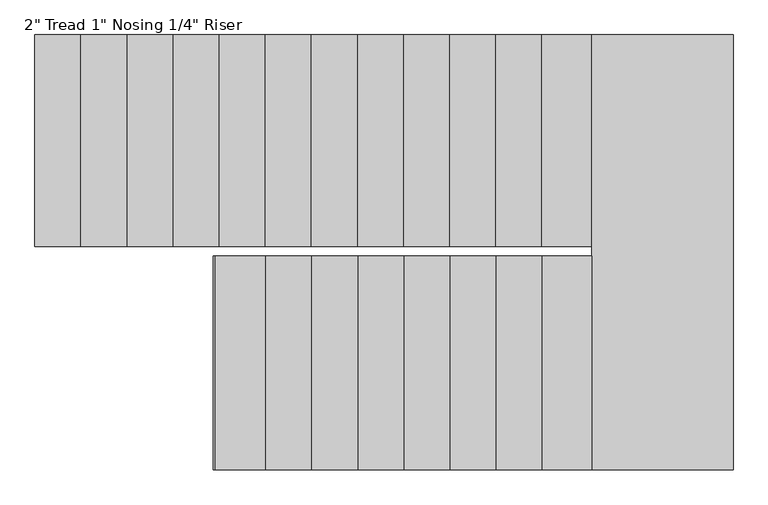
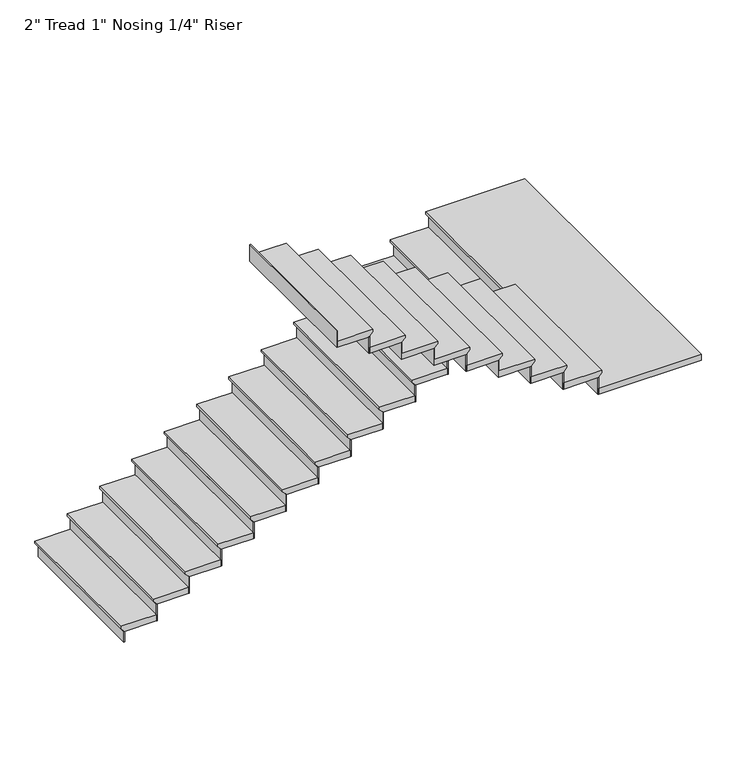
"""IFC4 building model written with IfcOpenShell, lengths in millimetres: stair flight geometry."""

from ifc_helpers import new_model, si_unit, origin, place, context, project, spatial, faceted_brep, source, transform, mapped, element, save


def stair_flight_4668eb62(model_context):
    return source(origin(), model_context, "Body", "Brep", [
        faceted_brep([(1811.8890963, 296.3962251, 6215.4954545), (1811.8890963, 296.3962251, 6234.5454545), (1811.8890963, 1464.7962251, 6234.5454545), (1811.8890963, 1464.7962251, 6215.4954545), (1837.2890963, 296.3962251, 6190.0954545), (1837.2890963, 1464.7962251, 6190.0954545), (2091.2890963, 296.3962251, 6234.5454545), (2091.2890963, 1464.7962251, 6234.5454545), (1837.2890963, 1464.7962251, 6183.7454545), (2091.2890963, 1464.7962251, 6183.7454545), (2091.2890963, 296.3962251, 6183.7454545), (1837.2890963, 296.3962251, 6183.7454545)], [[[0, 1, 2, 3]], [[4, 0, 3, 5]], [[2, 1, 6, 7]], [[8, 9, 10, 11]], [[2, 7, 9, 8, 5, 3]], [[8, 11, 4, 5]], [[6, 1, 0, 4, 11, 10]], [[7, 6, 10, 9]]]),
        faceted_brep([(1837.2890963, 296.3962251, 6183.7454545), (1837.2890963, 296.3962251, 6096.0), (1843.6390963, 296.3962251, 6096.0), (1843.6390963, 296.3962251, 6183.7454545), (1837.2890963, 1464.7962251, 6183.7454545), (1843.6390963, 1464.7962251, 6183.7454545), (1843.6390963, 1464.7962251, 6096.0), (1837.2890963, 1464.7962251, 6096.0)], [[[0, 1, 2, 3]], [[4, 5, 6, 7]], [[1, 0, 4, 7]], [[2, 1, 7, 6]], [[3, 2, 6, 5]], [[0, 3, 5, 4]]]),
        faceted_brep([(2091.2890963, 296.3962251, 6322.2909091), (2091.2890963, 296.3962251, 6183.7454545), (2097.6390963, 296.3962251, 6183.7454545), (2097.6390963, 296.3962251, 6322.2909091), (2091.2890963, 1464.7962251, 6322.2909091), (2097.6390963, 1464.7962251, 6322.2909091), (2097.6390963, 1464.7962251, 6183.7454545), (2091.2890963, 1464.7962251, 6183.7454545)], [[[0, 1, 2, 3]], [[4, 5, 6, 7]], [[1, 0, 4, 7]], [[2, 1, 7, 6]], [[3, 2, 6, 5]], [[0, 3, 5, 4]]]),
        faceted_brep([(2065.8890963, 1464.7962251, 6373.0909091), (2065.8890963, 296.3962251, 6373.0909091), (2345.2890963, 296.3962251, 6373.0909091), (2345.2890963, 1464.7962251, 6373.0909091), (2091.2890963, 1464.7962251, 6322.2909091), (2345.2890963, 1464.7962251, 6322.2909091), (2345.2890963, 296.3962251, 6322.2909091), (2091.2890963, 296.3962251, 6322.2909091), (2091.2890963, 1464.7962251, 6328.6409091), (2065.8890963, 1464.7962251, 6354.0409091), (2091.2890963, 296.3962251, 6328.6409091), (2065.8890963, 296.3962251, 6354.0409091)], [[[0, 1, 2, 3]], [[4, 5, 6, 7]], [[0, 3, 5, 4, 8, 9]], [[4, 7, 10, 8]], [[2, 1, 11, 10, 7, 6]], [[3, 2, 6, 5]], [[11, 1, 0, 9]], [[10, 11, 9, 8]]]),
        faceted_brep([(2345.2890963, 296.3962251, 6460.8363636), (2345.2890963, 296.3962251, 6322.2909091), (2351.6390963, 296.3962251, 6322.2909091), (2351.6390963, 296.3962251, 6460.8363636), (2345.2890963, 1464.7962251, 6460.8363636), (2351.6390963, 1464.7962251, 6460.8363636), (2351.6390963, 1464.7962251, 6322.2909091), (2345.2890963, 1464.7962251, 6322.2909091)], [[[0, 1, 2, 3]], [[4, 5, 6, 7]], [[1, 0, 4, 7]], [[2, 1, 7, 6]], [[3, 2, 6, 5]], [[0, 3, 5, 4]]]),
        faceted_brep([(2319.8890963, 1464.7962251, 6511.6363636), (2319.8890963, 296.3962251, 6511.6363636), (2599.2890963, 296.3962251, 6511.6363636), (2599.2890963, 1464.7962251, 6511.6363636), (2345.2890963, 1464.7962251, 6460.8363636), (2599.2890963, 1464.7962251, 6460.8363636), (2599.2890963, 296.3962251, 6460.8363636), (2345.2890963, 296.3962251, 6460.8363636), (2345.2890963, 1464.7962251, 6467.1863636), (2319.8890963, 1464.7962251, 6492.5863636), (2345.2890963, 296.3962251, 6467.1863636), (2319.8890963, 296.3962251, 6492.5863636)], [[[0, 1, 2, 3]], [[4, 5, 6, 7]], [[0, 3, 5, 4, 8, 9]], [[4, 7, 10, 8]], [[2, 1, 11, 10, 7, 6]], [[3, 2, 6, 5]], [[11, 1, 0, 9]], [[10, 11, 9, 8]]]),
        faceted_brep([(2599.2890963, 296.3962251, 6599.3818182), (2599.2890963, 296.3962251, 6460.8363636), (2605.6390963, 296.3962251, 6460.8363636), (2605.6390963, 296.3962251, 6599.3818182), (2599.2890963, 1464.7962251, 6599.3818182), (2605.6390963, 1464.7962251, 6599.3818182), (2605.6390963, 1464.7962251, 6460.8363636), (2599.2890963, 1464.7962251, 6460.8363636)], [[[0, 1, 2, 3]], [[4, 5, 6, 7]], [[1, 0, 4, 7]], [[2, 1, 7, 6]], [[3, 2, 6, 5]], [[0, 3, 5, 4]]]),
        faceted_brep([(2573.8890963, 1464.7962251, 6650.1818182), (2573.8890963, 296.3962251, 6650.1818182), (2853.2890963, 296.3962251, 6650.1818182), (2853.2890963, 1464.7962251, 6650.1818182), (2599.2890963, 1464.7962251, 6599.3818182), (2853.2890963, 1464.7962251, 6599.3818182), (2853.2890963, 296.3962251, 6599.3818182), (2599.2890963, 296.3962251, 6599.3818182), (2599.2890963, 1464.7962251, 6605.7318182), (2573.8890963, 1464.7962251, 6631.1318182), (2599.2890963, 296.3962251, 6605.7318182), (2573.8890963, 296.3962251, 6631.1318182)], [[[0, 1, 2, 3]], [[4, 5, 6, 7]], [[0, 3, 5, 4, 8, 9]], [[4, 7, 10, 8]], [[2, 1, 11, 10, 7, 6]], [[3, 2, 6, 5]], [[11, 1, 0, 9]], [[10, 11, 9, 8]]]),
        faceted_brep([(2853.2890963, 296.3962251, 6737.9272727), (2853.2890963, 296.3962251, 6599.3818182), (2859.6390963, 296.3962251, 6599.3818182), (2859.6390963, 296.3962251, 6737.9272727), (2853.2890963, 1464.7962251, 6737.9272727), (2859.6390963, 1464.7962251, 6737.9272727), (2859.6390963, 1464.7962251, 6599.3818182), (2853.2890963, 1464.7962251, 6599.3818182)], [[[0, 1, 2, 3]], [[4, 5, 6, 7]], [[1, 0, 4, 7]], [[2, 1, 7, 6]], [[3, 2, 6, 5]], [[0, 3, 5, 4]]]),
        faceted_brep([(2827.8890963, 1464.7962251, 6788.7272727), (2827.8890963, 296.3962251, 6788.7272727), (3107.2890963, 296.3962251, 6788.7272727), (3107.2890963, 1464.7962251, 6788.7272727), (2853.2890963, 1464.7962251, 6737.9272727), (3107.2890963, 1464.7962251, 6737.9272727), (3107.2890963, 296.3962251, 6737.9272727), (2853.2890963, 296.3962251, 6737.9272727), (2853.2890963, 1464.7962251, 6744.2772727), (2827.8890963, 1464.7962251, 6769.6772727), (2853.2890963, 296.3962251, 6744.2772727), (2827.8890963, 296.3962251, 6769.6772727)], [[[0, 1, 2, 3]], [[4, 5, 6, 7]], [[0, 3, 5, 4, 8, 9]], [[4, 7, 10, 8]], [[2, 1, 11, 10, 7, 6]], [[3, 2, 6, 5]], [[11, 1, 0, 9]], [[10, 11, 9, 8]]]),
        faceted_brep([(3107.2890963, 296.3962251, 6876.4727273), (3107.2890963, 296.3962251, 6737.9272727), (3113.6390963, 296.3962251, 6737.9272727), (3113.6390963, 296.3962251, 6876.4727273), (3107.2890963, 1464.7962251, 6876.4727273), (3113.6390963, 1464.7962251, 6876.4727273), (3113.6390963, 1464.7962251, 6737.9272727), (3107.2890963, 1464.7962251, 6737.9272727)], [[[0, 1, 2, 3]], [[4, 5, 6, 7]], [[1, 0, 4, 7]], [[2, 1, 7, 6]], [[3, 2, 6, 5]], [[0, 3, 5, 4]]]),
        faceted_brep([(3081.8890963, 1464.7962251, 6927.2727273), (3081.8890963, 296.3962251, 6927.2727273), (3361.2890963, 296.3962251, 6927.2727273), (3361.2890963, 1464.7962251, 6927.2727273), (3107.2890963, 1464.7962251, 6876.4727273), (3361.2890963, 1464.7962251, 6876.4727273), (3361.2890963, 296.3962251, 6876.4727273), (3107.2890963, 296.3962251, 6876.4727273), (3107.2890963, 1464.7962251, 6882.8227273), (3081.8890963, 1464.7962251, 6908.2227273), (3107.2890963, 296.3962251, 6882.8227273), (3081.8890963, 296.3962251, 6908.2227273)], [[[0, 1, 2, 3]], [[4, 5, 6, 7]], [[0, 3, 5, 4, 8, 9]], [[4, 7, 10, 8]], [[2, 1, 11, 10, 7, 6]], [[3, 2, 6, 5]], [[11, 1, 0, 9]], [[10, 11, 9, 8]]]),
        faceted_brep([(3361.2890963, 296.3962251, 7015.0181818), (3361.2890963, 296.3962251, 6876.4727273), (3367.6390963, 296.3962251, 6876.4727273), (3367.6390963, 296.3962251, 7015.0181818), (3361.2890963, 1464.7962251, 7015.0181818), (3367.6390963, 1464.7962251, 7015.0181818), (3367.6390963, 1464.7962251, 6876.4727273), (3361.2890963, 1464.7962251, 6876.4727273)], [[[0, 1, 2, 3]], [[4, 5, 6, 7]], [[1, 0, 4, 7]], [[2, 1, 7, 6]], [[3, 2, 6, 5]], [[0, 3, 5, 4]]]),
        faceted_brep([(3335.8890963, 1464.7962251, 7065.8181818), (3335.8890963, 296.3962251, 7065.8181818), (3615.2890963, 296.3962251, 7065.8181818), (3615.2890963, 1464.7962251, 7065.8181818), (3361.2890963, 1464.7962251, 7015.0181818), (3615.2890963, 1464.7962251, 7015.0181818), (3615.2890963, 296.3962251, 7015.0181818), (3361.2890963, 296.3962251, 7015.0181818), (3361.2890963, 1464.7962251, 7021.3681818), (3335.8890963, 1464.7962251, 7046.7681818), (3361.2890963, 296.3962251, 7021.3681818), (3335.8890963, 296.3962251, 7046.7681818)], [[[0, 1, 2, 3]], [[4, 5, 6, 7]], [[0, 3, 5, 4, 8, 9]], [[4, 7, 10, 8]], [[2, 1, 11, 10, 7, 6]], [[3, 2, 6, 5]], [[11, 1, 0, 9]], [[10, 11, 9, 8]]]),
        faceted_brep([(3615.2890963, 296.3962251, 7153.5636364), (3615.2890963, 296.3962251, 7015.0181818), (3621.6390963, 296.3962251, 7015.0181818), (3621.6390963, 296.3962251, 7153.5636364), (3615.2890963, 1464.7962251, 7153.5636364), (3621.6390963, 1464.7962251, 7153.5636364), (3621.6390963, 1464.7962251, 7015.0181818), (3615.2890963, 1464.7962251, 7015.0181818)], [[[0, 1, 2, 3]], [[4, 5, 6, 7]], [[1, 0, 4, 7]], [[2, 1, 7, 6]], [[3, 2, 6, 5]], [[0, 3, 5, 4]]]),
        faceted_brep([(3589.8890963, 1464.7962251, 7204.3636364), (3589.8890963, 296.3962251, 7204.3636364), (3869.2890963, 296.3962251, 7204.3636364), (3869.2890963, 1464.7962251, 7204.3636364), (3615.2890963, 1464.7962251, 7153.5636364), (3869.2890963, 1464.7962251, 7153.5636364), (3869.2890963, 296.3962251, 7153.5636364), (3615.2890963, 296.3962251, 7153.5636364), (3615.2890963, 1464.7962251, 7159.9136364), (3589.8890963, 1464.7962251, 7185.3136364), (3615.2890963, 296.3962251, 7159.9136364), (3589.8890963, 296.3962251, 7185.3136364)], [[[0, 1, 2, 3]], [[4, 5, 6, 7]], [[0, 3, 5, 4, 8, 9]], [[4, 7, 10, 8]], [[2, 1, 11, 10, 7, 6]], [[3, 2, 6, 5]], [[11, 1, 0, 9]], [[10, 11, 9, 8]]]),
        faceted_brep([(3869.2890963, 296.3962251, 7292.1090909), (3869.2890963, 296.3962251, 7153.5636364), (3875.6390963, 296.3962251, 7153.5636364), (3875.6390963, 296.3962251, 7292.1090909), (3869.2890963, 1464.7962251, 7292.1090909), (3875.6390963, 1464.7962251, 7292.1090909), (3875.6390963, 1464.7962251, 7153.5636364), (3869.2890963, 1464.7962251, 7153.5636364)], [[[0, 1, 2, 3]], [[4, 5, 6, 7]], [[1, 0, 4, 7]], [[2, 1, 7, 6]], [[3, 2, 6, 5]], [[0, 3, 5, 4]]]),
        faceted_brep([(3843.8890963, 1464.7962251, 7342.9090909), (3843.8890963, 296.3962251, 7342.9090909), (4123.2890963, 296.3962251, 7342.9090909), (4123.2890963, 1464.7962251, 7342.9090909), (3869.2890963, 1464.7962251, 7292.1090909), (4123.2890963, 1464.7962251, 7292.1090909), (4123.2890963, 296.3962251, 7292.1090909), (3869.2890963, 296.3962251, 7292.1090909), (3869.2890963, 1464.7962251, 7298.4590909), (3843.8890963, 1464.7962251, 7323.8590909), (3869.2890963, 296.3962251, 7298.4590909), (3843.8890963, 296.3962251, 7323.8590909)], [[[0, 1, 2, 3]], [[4, 5, 6, 7]], [[0, 3, 5, 4, 8, 9]], [[4, 7, 10, 8]], [[2, 1, 11, 10, 7, 6]], [[3, 2, 6, 5]], [[11, 1, 0, 9]], [[10, 11, 9, 8]]]),
        faceted_brep([(4123.2890963, 296.3962251, 7430.6545455), (4123.2890963, 296.3962251, 7292.1090909), (4129.6390963, 296.3962251, 7292.1090909), (4129.6390963, 296.3962251, 7430.6545455), (4123.2890963, 1464.7962251, 7430.6545455), (4129.6390963, 1464.7962251, 7430.6545455), (4129.6390963, 1464.7962251, 7292.1090909), (4123.2890963, 1464.7962251, 7292.1090909)], [[[0, 1, 2, 3]], [[4, 5, 6, 7]], [[1, 0, 4, 7]], [[2, 1, 7, 6]], [[3, 2, 6, 5]], [[0, 3, 5, 4]]]),
        faceted_brep([(4097.8890963, 1464.7962251, 7481.4545455), (4097.8890963, 296.3962251, 7481.4545455), (4377.2890963, 296.3962251, 7481.4545455), (4377.2890963, 1464.7962251, 7481.4545455), (4123.2890963, 1464.7962251, 7430.6545455), (4377.2890963, 1464.7962251, 7430.6545455), (4377.2890963, 296.3962251, 7430.6545455), (4123.2890963, 296.3962251, 7430.6545455), (4123.2890963, 1464.7962251, 7437.0045455), (4097.8890963, 1464.7962251, 7462.4045455), (4123.2890963, 296.3962251, 7437.0045455), (4097.8890963, 296.3962251, 7462.4045455)], [[[0, 1, 2, 3]], [[4, 5, 6, 7]], [[0, 3, 5, 4, 8, 9]], [[4, 7, 10, 8]], [[2, 1, 11, 10, 7, 6]], [[3, 2, 6, 5]], [[11, 1, 0, 9]], [[10, 11, 9, 8]]]),
        faceted_brep([(4377.2890963, 296.3962251, 7569.2), (4377.2890963, 296.3962251, 7430.6545455), (4383.6390963, 296.3962251, 7430.6545455), (4383.6390963, 296.3962251, 7569.2), (4377.2890963, 1464.7962251, 7569.2), (4383.6390963, 1464.7962251, 7569.2), (4383.6390963, 1464.7962251, 7430.6545455), (4377.2890963, 1464.7962251, 7430.6545455)], [[[0, 1, 2, 3]], [[4, 5, 6, 7]], [[1, 0, 4, 7]], [[2, 1, 7, 6]], [[3, 2, 6, 5]], [[0, 3, 5, 4]]]),
        faceted_brep([(4351.8890963, 1464.7962251, 7620.0), (4351.8890963, 296.3962251, 7620.0), (4631.2890963, 296.3962251, 7620.0), (4631.2890963, 1464.7962251, 7620.0), (4377.2890963, 1464.7962251, 7569.2), (4631.2890963, 1464.7962251, 7569.2), (4631.2890963, 296.3962251, 7569.2), (4377.2890963, 296.3962251, 7569.2), (4377.2890963, 1464.7962251, 7575.55), (4351.8890963, 1464.7962251, 7600.95), (4377.2890963, 296.3962251, 7575.55), (4351.8890963, 296.3962251, 7600.95)], [[[0, 1, 2, 3]], [[4, 5, 6, 7]], [[0, 3, 5, 4, 8, 9]], [[4, 7, 10, 8]], [[2, 1, 11, 10, 7, 6]], [[3, 2, 6, 5]], [[11, 1, 0, 9]], [[10, 11, 9, 8]]]),
        faceted_brep([(4631.2890963, 296.3962251, 7707.7454545), (4631.2890963, 296.3962251, 7569.2), (4637.6390963, 296.3962251, 7569.2), (4637.6390963, 296.3962251, 7707.7454545), (4631.2890963, 1464.7962251, 7707.7454545), (4637.6390963, 1464.7962251, 7707.7454545), (4637.6390963, 1464.7962251, 7569.2), (4631.2890963, 1464.7962251, 7569.2)], [[[0, 1, 2, 3]], [[4, 5, 6, 7]], [[1, 0, 4, 7]], [[2, 1, 7, 6]], [[3, 2, 6, 5]], [[0, 3, 5, 4]]]),
        faceted_brep([(4605.8890963, 1464.7962251, 7758.5454545), (4605.8890963, 296.3962251, 7758.5454545), (4906.4326586, 296.3962251, 7758.5454545), (4906.4326586, 1464.7962251, 7758.5454545), (4631.2890963, 1464.7962251, 7707.7454545), (4906.4326586, 1464.7962251, 7707.7454545), (4906.4326586, 296.3962251, 7707.7454545), (4631.2890963, 296.3962251, 7707.7454545), (4631.2890963, 1464.7962251, 7714.0954545), (4605.8890963, 1464.7962251, 7739.4954545), (4631.2890963, 296.3962251, 7714.0954545), (4605.8890963, 296.3962251, 7739.4954545)], [[[0, 1, 2, 3]], [[4, 5, 6, 7]], [[0, 3, 5, 4, 8, 9]], [[4, 7, 10, 8]], [[2, 1, 11, 10, 7, 6]], [[3, 2, 6, 5]], [[11, 1, 0, 9]], [[10, 11, 9, 8]]]),
        faceted_brep([(4906.4326586, 296.3962251, 7846.2909091), (4906.4326586, 296.3962251, 7707.7454545), (4912.7826586, 296.3962251, 7707.7454545), (4912.7826586, 296.3962251, 7846.2909091), (4906.4326586, 1464.7962251, 7846.2909091), (4912.7826586, 1464.7962251, 7846.2909091), (4912.7826586, 1464.7962251, 7707.7454545), (4906.4326586, 1464.7962251, 7707.7454545)], [[[0, 1, 2, 3]], [[4, 5, 6, 7]], [[1, 0, 4, 7]], [[2, 1, 7, 6]], [[3, 2, 6, 5]], [[0, 3, 5, 4]]]),
        faceted_brep([(4855.6326586, -935.5037749, 7897.0909091), (5659.9890963, -935.5037749, 7897.0909091), (5659.9890963, 1464.7962251, 7897.0909091), (4881.0326586, 1464.7962251, 7897.0909091), (4881.0326586, 245.5962251, 7897.0909091), (4855.6326586, 245.5962251, 7897.0909091), (5659.9890963, -935.5037749, 7846.2909091), (4855.6326586, -935.5037749, 7846.2909091), (4855.6326586, 245.5962251, 7846.2909091), (4881.0326586, 245.5962251, 7846.2909091), (4881.0326586, 296.3962251, 7846.2909091), (4906.4326586, 296.3962251, 7846.2909091), (4906.4326586, 1464.7962251, 7846.2909091), (5659.9890963, 1464.7962251, 7846.2909091), (4906.4326586, 1464.7962251, 7852.6409091), (4881.0326586, 1464.7962251, 7878.0409091), (4906.4326586, 296.3962251, 7852.6409091), (4881.0326586, 296.3962251, 7878.0409091)], [[[0, 1, 2, 3, 4, 5]], [[6, 7, 8, 9, 10, 11, 12, 13]], [[1, 0, 7, 6]], [[2, 1, 6, 13]], [[3, 2, 13, 12, 14, 15]], [[12, 11, 16, 14]], [[11, 10, 17, 16]], [[4, 3, 15, 17, 10, 9]], [[5, 4, 9, 8]], [[0, 5, 8, 7]], [[15, 14, 16, 17]]]),
        faceted_brep([(4855.6326586, 245.5962251, 7984.8363636), (4855.6326586, 245.5962251, 7846.2909091), (4849.2826586, 245.5962251, 7846.2909091), (4849.2826586, 245.5962251, 7984.8363636), (4855.6326586, -935.5037749, 7984.8363636), (4849.2826586, -935.5037749, 7984.8363636), (4849.2826586, -935.5037749, 7846.2909091), (4855.6326586, -935.5037749, 7846.2909091)], [[[0, 1, 2, 3]], [[4, 5, 6, 7]], [[1, 0, 4, 7]], [[2, 1, 7, 6]], [[3, 2, 6, 5]], [[0, 3, 5, 4]]]),
        faceted_brep([(4881.0326586, -935.5037749, 8035.6363636), (4881.0326586, 245.5962251, 8035.6363636), (4580.4890963, 245.5962251, 8035.6363636), (4580.4890963, -935.5037749, 8035.6363636), (4855.6326586, -935.5037749, 7984.8363636), (4580.4890963, -935.5037749, 7984.8363636), (4580.4890963, 245.5962251, 7984.8363636), (4855.6326586, 245.5962251, 7984.8363636), (4855.6326586, -935.5037749, 7991.1863636), (4881.0326586, -935.5037749, 8016.5863636), (4855.6326586, 245.5962251, 7991.1863636), (4881.0326586, 245.5962251, 8016.5863636)], [[[0, 1, 2, 3]], [[4, 5, 6, 7]], [[0, 3, 5, 4, 8, 9]], [[4, 7, 10, 8]], [[2, 1, 11, 10, 7, 6]], [[3, 2, 6, 5]], [[11, 1, 0, 9]], [[10, 11, 9, 8]]]),
        faceted_brep([(4580.4890963, 245.5962251, 8123.3818182), (4580.4890963, 245.5962251, 7984.8363636), (4574.1390963, 245.5962251, 7984.8363636), (4574.1390963, 245.5962251, 8123.3818182), (4580.4890963, -935.5037749, 8123.3818182), (4574.1390963, -935.5037749, 8123.3818182), (4574.1390963, -935.5037749, 7984.8363636), (4580.4890963, -935.5037749, 7984.8363636)], [[[0, 1, 2, 3]], [[4, 5, 6, 7]], [[1, 0, 4, 7]], [[2, 1, 7, 6]], [[3, 2, 6, 5]], [[0, 3, 5, 4]]]),
        faceted_brep([(4605.8890963, -935.5037749, 8174.1818182), (4605.8890963, 245.5962251, 8174.1818182), (4326.4890963, 245.5962251, 8174.1818182), (4326.4890963, -935.5037749, 8174.1818182), (4580.4890963, -935.5037749, 8123.3818182), (4326.4890963, -935.5037749, 8123.3818182), (4326.4890963, 245.5962251, 8123.3818182), (4580.4890963, 245.5962251, 8123.3818182), (4580.4890963, -935.5037749, 8129.7318182), (4605.8890963, -935.5037749, 8155.1318182), (4580.4890963, 245.5962251, 8129.7318182), (4605.8890963, 245.5962251, 8155.1318182)], [[[0, 1, 2, 3]], [[4, 5, 6, 7]], [[0, 3, 5, 4, 8, 9]], [[4, 7, 10, 8]], [[2, 1, 11, 10, 7, 6]], [[3, 2, 6, 5]], [[11, 1, 0, 9]], [[10, 11, 9, 8]]]),
        faceted_brep([(4326.4890963, 245.5962251, 8261.9272727), (4326.4890963, 245.5962251, 8123.3818182), (4320.1390963, 245.5962251, 8123.3818182), (4320.1390963, 245.5962251, 8261.9272727), (4326.4890963, -935.5037749, 8261.9272727), (4320.1390963, -935.5037749, 8261.9272727), (4320.1390963, -935.5037749, 8123.3818182), (4326.4890963, -935.5037749, 8123.3818182)], [[[0, 1, 2, 3]], [[4, 5, 6, 7]], [[1, 0, 4, 7]], [[2, 1, 7, 6]], [[3, 2, 6, 5]], [[0, 3, 5, 4]]]),
        faceted_brep([(4351.8890963, -935.5037749, 8312.7272727), (4351.8890963, 245.5962251, 8312.7272727), (4072.4890963, 245.5962251, 8312.7272727), (4072.4890963, -935.5037749, 8312.7272727), (4326.4890963, -935.5037749, 8261.9272727), (4072.4890963, -935.5037749, 8261.9272727), (4072.4890963, 245.5962251, 8261.9272727), (4326.4890963, 245.5962251, 8261.9272727), (4326.4890963, -935.5037749, 8268.2772727), (4351.8890963, -935.5037749, 8293.6772727), (4326.4890963, 245.5962251, 8268.2772727), (4351.8890963, 245.5962251, 8293.6772727)], [[[0, 1, 2, 3]], [[4, 5, 6, 7]], [[0, 3, 5, 4, 8, 9]], [[4, 7, 10, 8]], [[2, 1, 11, 10, 7, 6]], [[3, 2, 6, 5]], [[11, 1, 0, 9]], [[10, 11, 9, 8]]]),
        faceted_brep([(4072.4890963, 245.5962251, 8400.4727273), (4072.4890963, 245.5962251, 8261.9272727), (4066.1390963, 245.5962251, 8261.9272727), (4066.1390963, 245.5962251, 8400.4727273), (4072.4890963, -935.5037749, 8400.4727273), (4066.1390963, -935.5037749, 8400.4727273), (4066.1390963, -935.5037749, 8261.9272727), (4072.4890963, -935.5037749, 8261.9272727)], [[[0, 1, 2, 3]], [[4, 5, 6, 7]], [[1, 0, 4, 7]], [[2, 1, 7, 6]], [[3, 2, 6, 5]], [[0, 3, 5, 4]]]),
        faceted_brep([(4097.8890963, -935.5037749, 8451.2727273), (4097.8890963, 245.5962251, 8451.2727273), (3818.4890963, 245.5962251, 8451.2727273), (3818.4890963, -935.5037749, 8451.2727273), (4072.4890963, -935.5037749, 8400.4727273), (3818.4890963, -935.5037749, 8400.4727273), (3818.4890963, 245.5962251, 8400.4727273), (4072.4890963, 245.5962251, 8400.4727273), (4072.4890963, -935.5037749, 8406.8227273), (4097.8890963, -935.5037749, 8432.2227273), (4072.4890963, 245.5962251, 8406.8227273), (4097.8890963, 245.5962251, 8432.2227273)], [[[0, 1, 2, 3]], [[4, 5, 6, 7]], [[0, 3, 5, 4, 8, 9]], [[4, 7, 10, 8]], [[2, 1, 11, 10, 7, 6]], [[3, 2, 6, 5]], [[11, 1, 0, 9]], [[10, 11, 9, 8]]]),
        faceted_brep([(3818.4890963, 245.5962251, 8539.0181818), (3818.4890963, 245.5962251, 8400.4727273), (3812.1390963, 245.5962251, 8400.4727273), (3812.1390963, 245.5962251, 8539.0181818), (3818.4890963, -935.5037749, 8539.0181818), (3812.1390963, -935.5037749, 8539.0181818), (3812.1390963, -935.5037749, 8400.4727273), (3818.4890963, -935.5037749, 8400.4727273)], [[[0, 1, 2, 3]], [[4, 5, 6, 7]], [[1, 0, 4, 7]], [[2, 1, 7, 6]], [[3, 2, 6, 5]], [[0, 3, 5, 4]]]),
        faceted_brep([(3843.8890963, -935.5037749, 8589.8181818), (3843.8890963, 245.5962251, 8589.8181818), (3564.4890963, 245.5962251, 8589.8181818), (3564.4890963, -935.5037749, 8589.8181818), (3818.4890963, -935.5037749, 8539.0181818), (3564.4890963, -935.5037749, 8539.0181818), (3564.4890963, 245.5962251, 8539.0181818), (3818.4890963, 245.5962251, 8539.0181818), (3818.4890963, -935.5037749, 8545.3681818), (3843.8890963, -935.5037749, 8570.7681818), (3818.4890963, 245.5962251, 8545.3681818), (3843.8890963, 245.5962251, 8570.7681818)], [[[0, 1, 2, 3]], [[4, 5, 6, 7]], [[0, 3, 5, 4, 8, 9]], [[4, 7, 10, 8]], [[2, 1, 11, 10, 7, 6]], [[3, 2, 6, 5]], [[11, 1, 0, 9]], [[10, 11, 9, 8]]]),
        faceted_brep([(3564.4890963, 245.5962251, 8677.5636364), (3564.4890963, 245.5962251, 8539.0181818), (3558.1390963, 245.5962251, 8539.0181818), (3558.1390963, 245.5962251, 8677.5636364), (3564.4890963, -935.5037749, 8677.5636364), (3558.1390963, -935.5037749, 8677.5636364), (3558.1390963, -935.5037749, 8539.0181818), (3564.4890963, -935.5037749, 8539.0181818)], [[[0, 1, 2, 3]], [[4, 5, 6, 7]], [[1, 0, 4, 7]], [[2, 1, 7, 6]], [[3, 2, 6, 5]], [[0, 3, 5, 4]]]),
        faceted_brep([(3589.8890963, -935.5037749, 8728.3636364), (3589.8890963, 245.5962251, 8728.3636364), (3310.4890963, 245.5962251, 8728.3636364), (3310.4890963, -935.5037749, 8728.3636364), (3564.4890963, -935.5037749, 8677.5636364), (3310.4890963, -935.5037749, 8677.5636364), (3310.4890963, 245.5962251, 8677.5636364), (3564.4890963, 245.5962251, 8677.5636364), (3564.4890963, -935.5037749, 8683.9136364), (3589.8890963, -935.5037749, 8709.3136364), (3564.4890963, 245.5962251, 8683.9136364), (3589.8890963, 245.5962251, 8709.3136364)], [[[0, 1, 2, 3]], [[4, 5, 6, 7]], [[0, 3, 5, 4, 8, 9]], [[4, 7, 10, 8]], [[2, 1, 11, 10, 7, 6]], [[3, 2, 6, 5]], [[11, 1, 0, 9]], [[10, 11, 9, 8]]]),
        faceted_brep([(3310.4890963, 245.5962251, 8816.1090909), (3310.4890963, 245.5962251, 8677.5636364), (3304.1390963, 245.5962251, 8677.5636364), (3304.1390963, 245.5962251, 8816.1090909), (3310.4890963, -935.5037749, 8816.1090909), (3304.1390963, -935.5037749, 8816.1090909), (3304.1390963, -935.5037749, 8677.5636364), (3310.4890963, -935.5037749, 8677.5636364)], [[[0, 1, 2, 3]], [[4, 5, 6, 7]], [[1, 0, 4, 7]], [[2, 1, 7, 6]], [[3, 2, 6, 5]], [[0, 3, 5, 4]]]),
        faceted_brep([(3335.8890963, -935.5037749, 8866.9090909), (3335.8890963, 245.5962251, 8866.9090909), (3056.4890963, 245.5962251, 8866.9090909), (3056.4890963, -935.5037749, 8866.9090909), (3310.4890963, -935.5037749, 8816.1090909), (3056.4890963, -935.5037749, 8816.1090909), (3056.4890963, 245.5962251, 8816.1090909), (3310.4890963, 245.5962251, 8816.1090909), (3310.4890963, -935.5037749, 8822.4590909), (3335.8890963, -935.5037749, 8847.8590909), (3310.4890963, 245.5962251, 8822.4590909), (3335.8890963, 245.5962251, 8847.8590909)], [[[0, 1, 2, 3]], [[4, 5, 6, 7]], [[0, 3, 5, 4, 8, 9]], [[4, 7, 10, 8]], [[2, 1, 11, 10, 7, 6]], [[3, 2, 6, 5]], [[11, 1, 0, 9]], [[10, 11, 9, 8]]]),
        faceted_brep([(3056.4890963, 245.5962251, 8954.6545455), (3056.4890963, 245.5962251, 8816.1090909), (3050.1390963, 245.5962251, 8816.1090909), (3050.1390963, 245.5962251, 8954.6545455), (3056.4890963, -935.5037749, 8954.6545455), (3050.1390963, -935.5037749, 8954.6545455), (3050.1390963, -935.5037749, 8816.1090909), (3056.4890963, -935.5037749, 8816.1090909)], [[[0, 1, 2, 3]], [[4, 5, 6, 7]], [[1, 0, 4, 7]], [[2, 1, 7, 6]], [[3, 2, 6, 5]], [[0, 3, 5, 4]]]),
        faceted_brep([(2802.4890963, 245.5962251, 9093.2), (2802.4890963, 245.5962251, 8954.6545455), (2796.1390963, 245.5962251, 8954.6545455), (2796.1390963, 245.5962251, 9093.2), (2802.4890963, -935.5037749, 9093.2), (2796.1390963, -935.5037749, 9093.2), (2796.1390963, -935.5037749, 8954.6545455), (2802.4890963, -935.5037749, 8954.6545455)], [[[0, 1, 2, 3]], [[4, 5, 6, 7]], [[1, 0, 4, 7]], [[2, 1, 7, 6]], [[3, 2, 6, 5]], [[0, 3, 5, 4]]]),
        faceted_brep([(3081.8890963, -935.5037749, 9005.4545455), (3081.8890963, 245.5962251, 9005.4545455), (2802.4890963, 245.5962251, 9005.4545455), (2802.4890963, -935.5037749, 9005.4545455), (3056.4890963, -935.5037749, 8954.6545455), (2802.4890963, -935.5037749, 8954.6545455), (2802.4890963, 245.5962251, 8954.6545455), (3056.4890963, 245.5962251, 8954.6545455), (3056.4890963, -935.5037749, 8961.0045455), (3081.8890963, -935.5037749, 8986.4045455), (3056.4890963, 245.5962251, 8961.0045455), (3081.8890963, 245.5962251, 8986.4045455)], [[[0, 1, 2, 3]], [[4, 5, 6, 7]], [[0, 3, 5, 4, 8, 9]], [[4, 7, 10, 8]], [[2, 1, 11, 10, 7, 6]], [[3, 2, 6, 5]], [[11, 1, 0, 9]], [[10, 11, 9, 8]]]),
    ])


if __name__ == "__main__":
    model = new_model("IFC4")
    model_context = context("Model", 3, world=origin())
    ifc_project = project(units=[si_unit("LENGTHUNIT", "METRE", prefix="MILLI")], contexts=[model_context])
    site = spatial("IfcSite", under=ifc_project)
    building = spatial("IfcBuilding", under=site)
    placement = place(None, origin())
    stair_flight_shape = stair_flight_4668eb62(model_context)
    element("IfcStairFlight", 1, ObjectType="2\" Tread 1\" Nosing 1/4\" Riser", at=placement, inside=building, context=model_context, shape_type="MappedRepresentation", body=[
        mapped(stair_flight_shape, transform((0.0, 0.0, 0.0), x_axis=(1.0, 0.0, 0.0), y_axis=(0.0, 1.0, 0.0), z_axis=(0.0, 0.0, 1.0))),
    ])
    save(model, "model.ifc")
